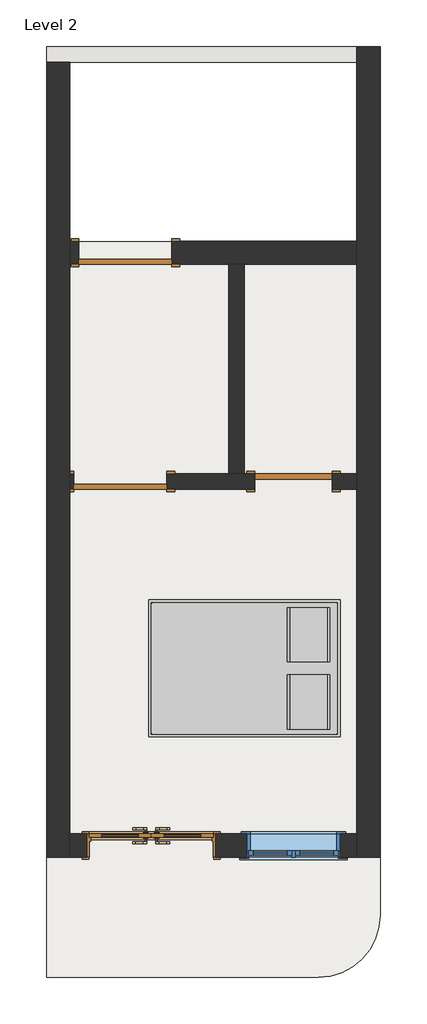
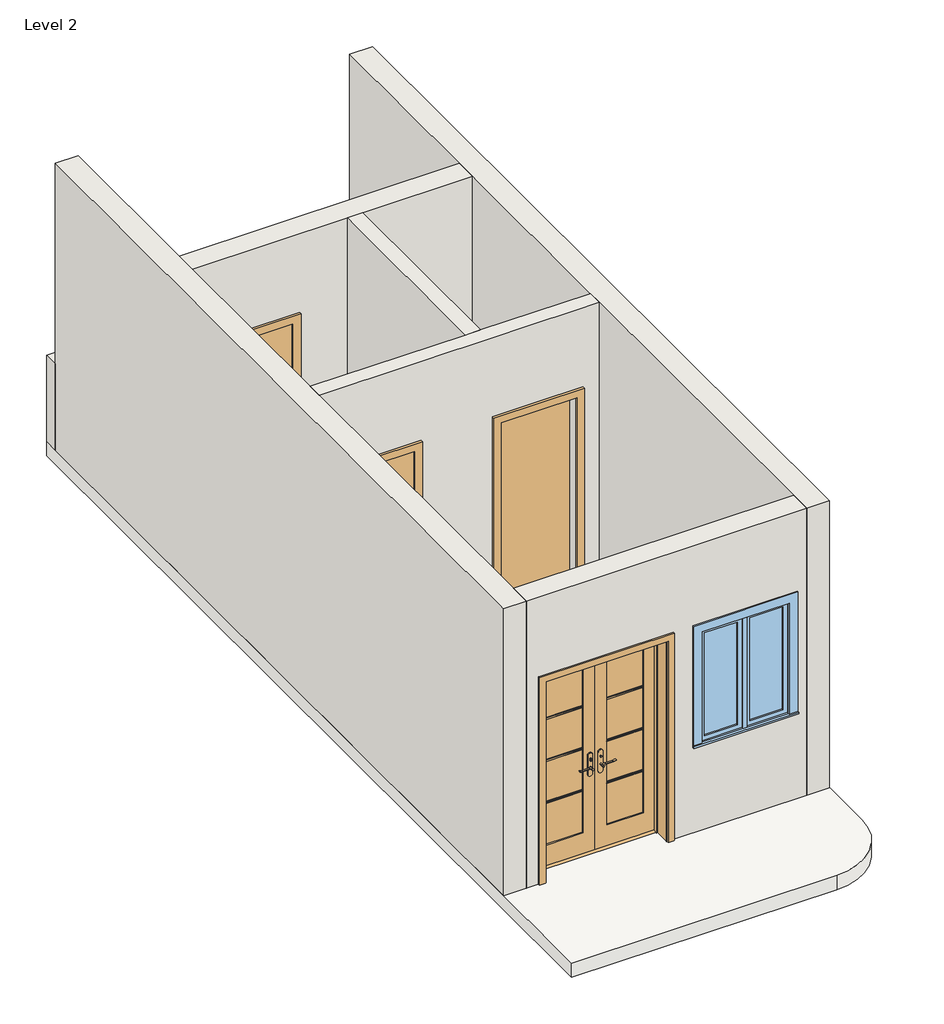
# One storey, incomplete: 7 walls, 4 doors, 1 furniture element, 1 slab, 1 window.
"""IFC4 building model written with IfcOpenShell, lengths in millimetres."""

from ifc_helpers import new_model, si_unit, point, frame, frame_2d, origin, place, context, project, spatial, polyline, circle_curve, trimmed, segment, composite_curve, outline, extrude, faceted_brep, transform, mapped, element, save
from components import door_4500b467, single_flush_2_5_e2b13fe9, door_0ca8825f, door_16372e1c, furniture_c8abb964, window_419b5846

model = new_model("IFC4")

# Units and contexts
model_context = context("Model", 3, world=origin())
ifc_project = project(units=[si_unit("LENGTHUNIT", "METRE", prefix="MILLI")], contexts=[model_context])

# Site, building, storey
site = spatial("IfcSite", under=ifc_project)
building = spatial("IfcBuilding", under=site)
storey = spatial("IfcBuildingStorey", under=building, Name="Level 2", Elevation=3200.4)

# Doors
placement = place(None, origin())
door_shape = door_4500b467(model_context)
element("IfcDoor", 1, ObjectType="Door-Exterior-Double-Full Glass-Wood_Clad : 48\" x 84\"", at=placement, inside=storey, context=model_context, shape_type="MappedRepresentation", body=[
    mapped(door_shape, transform((-5892.5189081, -995.9649972, 3200.4), x_axis=(1.0, 0.0, 0.0), y_axis=(0.0, 1.0, 0.0), z_axis=(0.0, 0.0, 1.0))),
])
single_flush_2_5_shape = single_flush_2_5_e2b13fe9(model_context)
element("IfcDoor", 2, ObjectType="Single-Flush : 2.5'", at=placement, inside=storey, context=model_context, shape_type="MappedRepresentation", body=[
    mapped(single_flush_2_5_shape, transform((-4495.5189081, 2575.9100028, 3200.4), x_axis=(-1.0, 0.0, 0.0), y_axis=(0.0, -1.0, 0.0), z_axis=(0.0, 0.0, 1.0))),
])
door_2_shape = door_0ca8825f(model_context)
element("IfcDoor", 3, ObjectType="Single-Flush : 36\" x 84\"", at=placement, inside=storey, context=model_context, shape_type="MappedRepresentation", body=[
    mapped(door_2_shape, transform((-6146.5189081, 4823.8100028, 3200.4), x_axis=(-1.0, 0.0, 0.0), y_axis=(0.0, -1.0, 0.0), z_axis=(0.0, 0.0, 1.0))),
])
door_3_shape = door_16372e1c(model_context)
element("IfcDoor", 4, ObjectType="Single-Flush : 36\" x 84\"", at=placement, inside=storey, context=model_context, shape_type="MappedRepresentation", body=[
    mapped(door_3_shape, transform((-6197.3189081, 2575.9100028, 3200.4), x_axis=(-1.0, 0.0, 0.0), y_axis=(0.0, -1.0, 0.0), z_axis=(0.0, 0.0, 1.0))),
])

# Furniture
furniture_shape = furniture_c8abb964(model_context)
element("IfcFurniture", 5, ObjectType="Bed-Box : Double 53\" x 74\"", at=placement, inside=storey, context=model_context, shape_type="MappedRepresentation", body=[
    mapped(furniture_shape, transform((-4743.6893999, 1079.9124618, 3200.4), x_axis=(0.0, -1.0000000000000002, 0.0), y_axis=(1.0000000000000002, 0.0, 0.0), z_axis=(0.0, 0.0, 1.0))),
])

# Slab
element("IfcSlab", 6, ObjectType="6\"", at=placement, inside=storey, context=model_context, shape_type="SweptSolid", body=[
    extrude(outline(composite_curve([segment(polyline([(-3644.6189081, 6849.4600028), (-3644.6189081, -1684.9399972)]), True, "CONTINUOUS"), segment(trimmed(circle_curve(frame_2d((-4254.2189081, -1684.9399972)), 609.6), [point((-3644.6189081, -1684.9399972))], [point((-4254.2189081, -2294.5399972))], False, "CARTESIAN"), True, "CONTINUOUS"), segment(polyline([(-4254.2189081, -2294.5399972), (-6921.2189081, -2294.5399972), (-6921.2189081, 6849.4600028), (-3644.6189081, 6849.4600028)]), True, "CONTINUOUS")], self_intersect=False), holes=[polyline([(-3873.2189081, 6697.0600028), (-6692.6189081, 6697.0600028), (-6692.6189081, 4938.1100028), (-3873.2189081, 4938.1100028), (-3873.2189081, 6697.0600028)])]), frame((0.0, 0.0, 3048.0), z_axis=(0.0, 0.0, 1.0), x_axis=(1.0, 0.0, 0.0)), (0.0, 0.0, 1.0), 152.4),
])

# Walls
element("IfcWall", 7, ObjectType="6\"", at=placement, inside=storey, context=model_context, shape_type="Brep", body=[
    faceted_brep([(-6921.2189081, 6697.0600028, 3200.4), (-6692.6189081, 6697.0600028, 3200.4), (-3873.2189081, 6697.0600028, 3200.4), (-3873.2189081, 6697.0600028, 4114.8), (-6921.2189081, 6697.0600028, 4114.8), (-6921.2189081, 6849.4600028, 3200.4), (-6921.2189081, 6849.4600028, 4114.8), (-3873.2189081, 6849.4600028, 4114.8), (-3873.2189081, 6849.4600028, 3200.4)], [[[0, 1, 2, 3, 4]], [[5, 6, 7, 8]], [[2, 1, 0, 5, 8]], [[4, 3, 7, 6]], [[0, 4, 6, 5]], [[3, 2, 8, 7]]]),
])
element("IfcWall", 8, ObjectType="6\"", at=placement, inside=storey, context=model_context, shape_type="Brep", body=[
    faceted_brep([(-6654.5189081, 2652.1100028, 5334.0), (-6654.5189081, 2652.1100028, 3200.4), (-6692.6189081, 2652.1100028, 3200.4), (-6692.6189081, 2652.1100028, 6248.4), (-5130.5189081, 2652.1100028, 6248.4), (-4978.1189081, 2652.1100028, 6248.4), (-3873.2189081, 2652.1100028, 6248.4), (-3873.2189081, 2652.1100028, 3200.4), (-4114.5189081, 2652.1100028, 3200.4), (-4114.5189081, 2652.1100028, 5334.0), (-4876.5189081, 2652.1100028, 5334.0), (-4876.5189081, 2652.1100028, 3200.4), (-4978.1189081, 2652.1100028, 3200.4), (-5130.5189081, 2652.1100028, 3200.4), (-5740.1189081, 2652.1100028, 3200.4), (-5740.1189081, 2652.1100028, 5334.0), (-6692.6189081, 2499.7100028, 3200.4), (-6654.5189081, 2499.7100028, 3200.4), (-6654.5189081, 2499.7100028, 5334.0), (-5740.1189081, 2499.7100028, 5334.0), (-5740.1189081, 2499.7100028, 3200.4), (-4876.5189081, 2499.7100028, 3200.4), (-4876.5189081, 2499.7100028, 5334.0), (-4114.5189081, 2499.7100028, 5334.0), (-4114.5189081, 2499.7100028, 3200.4), (-3873.2189081, 2499.7100028, 3200.4), (-3873.2189081, 2499.7100028, 6248.4), (-6692.6189081, 2499.7100028, 6248.4)], [[[0, 1, 2, 3, 4, 5, 6, 7, 8, 9, 10, 11, 12, 13, 14, 15]], [[16, 17, 18, 19, 20, 21, 22, 23, 24, 25, 26, 27]], [[8, 7, 25, 24]], [[2, 1, 17, 16]], [[14, 13, 12, 11, 21, 20]], [[6, 5, 4, 3, 27, 26]], [[3, 2, 16, 27]], [[7, 6, 26, 25]], [[22, 21, 11, 10]], [[23, 22, 10, 9]], [[24, 23, 9, 8]], [[18, 17, 1, 0]], [[19, 18, 0, 15]], [[20, 19, 15, 14]]]),
])
element("IfcWall", 9, ObjectType="6\"", at=placement, inside=storey, context=model_context, shape_type="SweptSolid", body=[
    extrude(outline(polyline([(-4978.1189081, 4709.5100028), (-4978.1189081, 2652.1100028), (-5130.5189081, 2652.1100028), (-5130.5189081, 4709.5100028), (-4978.1189081, 4709.5100028)])), frame((0.0, 0.0, 3200.4), z_axis=(0.0, 0.0, 1.0), x_axis=(1.0, 0.0, 0.0)), (0.0, 0.0, 1.0), 3048.0),
])
element("IfcWall", 10, ObjectType="9\"", at=placement, inside=storey, context=model_context, shape_type="Brep", body=[
    faceted_brep([(-3873.2189081, 6849.4600028, 3200.4), (-3873.2189081, 6697.0600028, 3200.4), (-3873.2189081, 4938.1100028, 3200.4), (-3873.2189081, 4709.5100028, 3200.4), (-3873.2189081, 2652.1100028, 3200.4), (-3873.2189081, 2499.7100028, 3200.4), (-3873.2189081, -884.8399972, 3200.4), (-3873.2189081, -1113.4399972, 3200.4), (-3873.2189081, -1113.4399972, 6248.4), (-3873.2189081, -884.8399972, 6248.4), (-3873.2189081, 2499.7100028, 6248.4), (-3873.2189081, 2652.1100028, 6248.4), (-3873.2189081, 4709.5100028, 6248.4), (-3873.2189081, 4938.1100028, 6248.4), (-3873.2189081, 6849.4600028, 6248.4), (-3873.2189081, 6849.4600028, 4114.8), (-3644.6189081, 6849.4600028, 3200.4), (-3644.6189081, 6849.4600028, 6248.4), (-3644.6189081, -1113.4399972, 6248.4), (-3644.6189081, -1113.4399972, 3200.4)], [[[0, 1, 2, 3, 4, 5, 6, 7, 8, 9, 10, 11, 12, 13, 14, 15]], [[16, 17, 18, 19]], [[7, 6, 5, 4, 3, 2, 1, 0, 16, 19]], [[14, 13, 12, 11, 10, 9, 8, 18, 17]], [[0, 15, 14, 17, 16]], [[8, 7, 19, 18]]]),
])
element("IfcWall", 11, ObjectType="9\"", at=placement, inside=storey, context=model_context, shape_type="Brep", body=[
    faceted_brep([(-6603.7189081, 4938.1100028, 5334.0), (-6603.7189081, 4938.1100028, 3200.4), (-6692.6189081, 4938.1100028, 3200.4), (-6692.6189081, 4938.1100028, 6248.4), (-3873.2189081, 4938.1100028, 6248.4), (-3873.2189081, 4938.1100028, 3200.4), (-5689.3189081, 4938.1100028, 3200.4), (-5689.3189081, 4938.1100028, 5334.0), (-6692.6189081, 4709.5100028, 3200.4), (-6603.7189081, 4709.5100028, 3200.4), (-6603.7189081, 4709.5100028, 5334.0), (-5689.3189081, 4709.5100028, 5334.0), (-5689.3189081, 4709.5100028, 3200.4), (-5130.5189081, 4709.5100028, 3200.4), (-4978.1189081, 4709.5100028, 3200.4), (-3873.2189081, 4709.5100028, 3200.4), (-3873.2189081, 4709.5100028, 6248.4), (-4978.1189081, 4709.5100028, 6248.4), (-5130.5189081, 4709.5100028, 6248.4), (-6692.6189081, 4709.5100028, 6248.4)], [[[0, 1, 2, 3, 4, 5, 6, 7]], [[8, 9, 10, 11, 12, 13, 14, 15, 16, 17, 18, 19]], [[6, 5, 15, 14, 13, 12]], [[2, 1, 9, 8]], [[4, 3, 19, 18, 17, 16]], [[3, 2, 8, 19]], [[5, 4, 16, 15]], [[10, 9, 1, 0]], [[11, 10, 0, 7]], [[12, 11, 7, 6]]]),
])
element("IfcWall", 12, ObjectType="9\"", at=placement, inside=storey, context=model_context, shape_type="SweptSolid", body=[
    extrude(outline(polyline([(6248.4, -3873.2189081), (6248.4, -6692.6189081), (3200.4, -6692.6189081), (3200.4, -6527.5189081), (5359.4, -6527.5189081), (5359.4, -5257.5189081), (3200.4, -5257.5189081), (3200.4, -3873.2189081), (6248.4, -3873.2189081)]), holes=[polyline([(5334.0, -4952.7189081), (5334.0, -4038.3189081), (4114.8, -4038.3189081), (4114.8, -4952.7189081), (5334.0, -4952.7189081)])]), frame((0.0, -1113.4399972, 0.0), z_axis=(0.0, 1.0, 0.0), x_axis=(0.0, 0.0, 1.0)), (0.0, 0.0, 1.0), 228.6),
])
element("IfcWall", 13, ObjectType="9\"", at=placement, inside=storey, context=model_context, shape_type="Brep", body=[
    faceted_brep([(-6692.6189081, -1113.4399972, 3200.4), (-6692.6189081, -884.8399972, 3200.4), (-6692.6189081, 2499.7100028, 3200.4), (-6692.6189081, 2652.1100028, 3200.4), (-6692.6189081, 4709.5100028, 3200.4), (-6692.6189081, 4938.1100028, 3200.4), (-6692.6189081, 6697.0600028, 3200.4), (-6692.6189081, 6697.0600028, 6248.4), (-6692.6189081, 4938.1100028, 6248.4), (-6692.6189081, 4709.5100028, 6248.4), (-6692.6189081, 2652.1100028, 6248.4), (-6692.6189081, 2499.7100028, 6248.4), (-6692.6189081, -884.8399972, 6248.4), (-6692.6189081, -1113.4399972, 6248.4), (-6921.2189081, -1113.4399972, 3200.4), (-6921.2189081, -1113.4399972, 6248.4), (-6921.2189081, 6697.0600028, 6248.4), (-6921.2189081, 6697.0600028, 4114.8), (-6921.2189081, 6697.0600028, 3200.4)], [[[0, 1, 2, 3, 4, 5, 6, 7, 8, 9, 10, 11, 12, 13]], [[14, 15, 16, 17, 18]], [[6, 5, 4, 3, 2, 1, 0, 14, 18]], [[13, 12, 11, 10, 9, 8, 7, 16, 15]], [[7, 6, 18, 17, 16]], [[0, 13, 15, 14]]]),
])

# Window
window_shape = window_419b5846(model_context)
element("IfcWindow", 14, ObjectType="Casement Dbl with Trim : 36\" x 48\"", at=placement, inside=storey, context=model_context, shape_type="MappedRepresentation", body=[
    mapped(window_shape, transform((-4495.5189081, -980.0899972, 3200.4), x_axis=(-1.0, 0.0, 0.0), y_axis=(0.0, -1.0, 0.0), z_axis=(0.0, 0.0, 1.0))),
])

save(model, "model.ifc")

# Revit data of these elements
# Type "Door-Exterior-Double-Full Glass-Wood_Clad : 48\" x 84\""
#   Type Mark = "9"
#   Assembly Code = "B2030100"
#   Analytic Construction = "French door, wood frame with double glass"
#   Top Rail = 0' - 4 11/16"
#   Threshold Offset [instance default] = 0' - 0 1/2"
#   Thickness = 0' - 1 3/8"
#   Thermal Resistance (R) = 1.9158 (h·ft²·°F)/BTU
#   Swing Angle [instance default] = 90.00°
#   Stiles = 0' - 4 3/4"
#   Rough Width = 4' - 2"
#   Rough Height = 7' - 1"
#   Panel Width = 2' - 0"
#   Door Offset [instance default] = 0' - 0"
#   Height = 7' - 0"
#   Width = 4' - 0"
#   Heat Transfer Coefficient (U) = 0.5220 BTU/(h·ft²·°F)
#   Bottom Rail = 0' - 9 1/8"
#   Exterior Trim [instance default] = yes
#   Threshold [instance default] = yes
#   Show Grill [instance default] = yes
#   Function = 1
#   Trim Material = Cherry
#   Threshold Material = Cherry
#   Panel Material = Cherry
#   Glazing = Glass
#   Frame Material = Cherry
#   Door Handle Material = Aluminum
#   Visual Light Transmittance = 0
#   Solar Heat Gain Coefficient = 0
#   Wall Closure = (empty or 0)
#   Construction Type = (empty or 0)
# Type "Single-Flush : 2.5'"
#   Type Mark = "8"
#   Construction Type Id = "MDOOR"
#   Assembly Code = "C1020"
#   Analytic Construction = "Metal"
#   Thickness = 0' - 2"
#   Heat Transfer Coefficient (U) = 0.651978 BTU/(h·ft²·°F)
#   Height = 7' - 0"
#   Trim Projection Ext = 0' - 1"
#   Trim Projection Int = 0' - 1"
#   Trim Width = 0' - 3"
#   Width = 2' - 6"
#   Define Thermal Properties by = 1
#   Door Material = Door - Panel
#   Frame Material = Door - Frame
#   Visual Light Transmittance = 0
#   Solar Heat Gain Coefficient = 0
#   Function = (empty or 0)
#   Wall Closure = (empty or 0)
# Type "Single-Flush : 36\" x 84\""
#   Type Mark = "1"
#   Construction Type Id = "MDOOR"
#   Assembly Code = "C1020"
#   Analytic Construction = "Metal"
#   Thickness = 0' - 2"
#   Heat Transfer Coefficient (U) = 0.651978 BTU/(h·ft²·°F)
#   Height = 7' - 0"
#   Trim Projection Ext = 0' - 1"
#   Trim Projection Int = 0' - 1"
#   Trim Width = 0' - 3"
#   Width = 3' - 0"
#   Define Thermal Properties by = 1
#   Door Material = Door - Panel
#   Frame Material = Door - Frame
#   Visual Light Transmittance = 0
#   Solar Heat Gain Coefficient = 0
#   Function = (empty or 0)
#   Wall Closure = (empty or 0)
# Type "Bed-Box : Double 53\" x 74\""
#   Assembly Code = "E2020200"
#   Length = 6' - 2"
#   Width = 4' - 5"
#   Frame Material = Birch
#   Mattress Material = Linen, White
#   Default Elevation = 0
# Type "6\""
#   Assembly Code = "B1010"
#   Function = 0
#   Layers, outside or top first: 0' - 6" no material (function 1)
# Type "6\""
#   Assembly Code = "B2010"
#   Layers, outside or top first: 0' - 6" no material (function 1)
# Type "9\""
#   Assembly Code = "B2010"
#   Layers, outside or top first: 0' - 9" no material (function 1)
# Type "Casement Dbl with Trim : 36\" x 48\""
#   Type Mark = "19"
#   Construction Type Id = "GSP4R"
#   Assembly Code = "B2020100"
#   Analytic Construction = "1/8 in Pilkington single glazing"
#   Visual Light Transmittance = 0.9
#   Solar Heat Gain Coefficient = 0.78
#   Heat Transfer Coefficient (U) = 0.6496 BTU/(h·ft²·°F)
#   Height = 4' - 0"
#   Default Sill Height = 3' - 0"
#   Trim Projection - Ext. = 0' - 0 1/2"
#   Trim Projection - Int. = 0' - 0 3/4"
#   Trim Width - Exterior = 0' - 3 1/2"
#   Trim Width - Interior = 0' - 3 1/2"
#   Width = 3' - 0"
#   Window Inset = 0' - 0 3/4"
#   Define Thermal Properties by = 1
#   Glass Pane Material = Glass
#   Sash Material = Sash
#   Trim Exterior Material = Trim
#   Trim Interior Material = Trim
#   Wall Closure = (empty or 0)
# Element 1 (IfcDoor, "Door-Exterior-Double-Full Glass-Wood_Clad : 48\" x 84\"")
#   Threshold Offset = 0' - 0 1/2"
#   Swing Angle = 90.00°
#   Door Offset = 0' - 0"
#   Threshold = yes
#   Show Grill = yes
#   Exterior Trim = yes
#   Phase Created = New Construction
#   Materials on its faces: "Cherry", "Aluminum", "Glass"
# Element 2 (IfcDoor, "Single-Flush : 2.5'")
#   Phase Created = New Construction
#   Materials on its faces: "Door - Frame", "Door - Panel"
# Elements 3, 4 (IfcDoor, "Single-Flush : 36\" x 84\"")
#   Phase Created = New Construction
#   Materials on its faces: "Door - Frame", "Door - Panel"
# Element 5 (IfcFurniture, "Bed-Box : Double 53\" x 74\"")
#   Phase Created = New Construction
#   Materials on its faces: "Birch", "Linen, White"
# Element 6 (IfcSlab, "6\"")
#   Height Offset From Level = 0' - 0"
#   Phase Created = New Construction
#   Materials on its faces: "Default Floor"
# Element 7 (IfcWall, "6\"")
#   Top Offset = 0' - 0"
#   Base Offset = 0' - 0"
#   Unconnected Height = 3' - 0"
#   wall height = 3' - 0"
#   Phase Created = New Construction
#   Base Constraint = Level 2
#   Materials on its faces: "Default Wall"
# Elements 8, 9 (IfcWall, "6\"")
#   Top Offset = 0' - 0"
#   Base Offset = 0' - 0"
#   Unconnected Height = 10' - 0"
#   wall height = 10' - 0"
#   Phase Created = New Construction
#   Base Constraint = Level 2
#   Materials on its faces: "Default Wall"
# Elements 10, 11, 12, 13 (IfcWall, "9\"")
#   Top Offset = 0' - 0"
#   Base Offset = 0' - 0"
#   Unconnected Height = 10' - 0"
#   wall height = 10' - 0"
#   Phase Created = New Construction
#   Base Constraint = Level 2
#   Materials on its faces: "Default Wall"
# Element 14 (IfcWindow, "Casement Dbl with Trim : 36\" x 48\"")
#   Mark = "1"
#   Phase Created = New Construction
#   Materials on its faces: "Sash", "Trim", "Glass"
# Materials
#   "Cherry": class "Wood", colour RGB 226 177 128, transparency 0, Description = "Prunus Serotina", Cost = 0
#   "Glass": class "Glass", colour RGB 0 128 192, transparency 0.75, Description = "Soda Lime Glass", Cost = 0
#   "Aluminum": class "Metal", colour RGB 247 247 247, transparency 0, Description = "Aluminum 6061", Cost = 0
#   "Door - Panel": class "Wood", colour RGB 210 159 95, transparency 0
#   "Door - Frame": colour RGB 118 70 51, transparency 0
#   "Birch": class "Wood", colour RGB 224 178 126, transparency 0, Description = "Betula Alleghaniensis", Cost = 0
#   "Linen, White": class "Textile", colour RGB 247 247 239, transparency 0, Description = "Linen, white", Cost = 0
#   "Sash": class "Wood", colour RGB 224 178 126, transparency 0
#   "Trim": class "Wood", colour RGB 224 178 126, transparency 0
#   "Default Floor": colour RGB 128 128 128, transparency 0
#   "Default Wall": colour RGB 128 128 128, transparency 0
